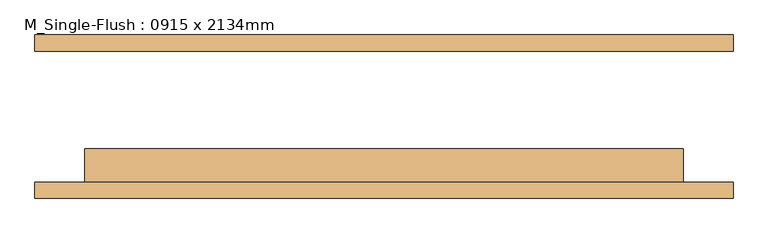
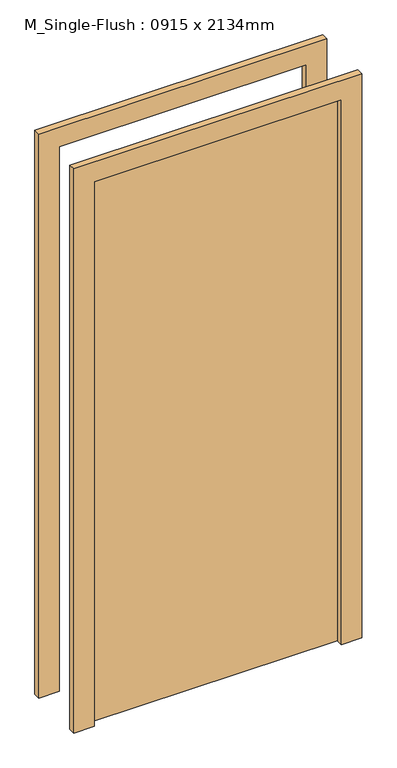
"""IFC4 building model written with IfcOpenShell, lengths in millimetres: door geometry, M_Single-Flush : 0915 x 2134mm."""

from ifc_helpers import new_model, si_unit, frame, origin, origin_with_axes, place, context, project, spatial, polyline, outline, extrude, source, transform, mapped, element, save


def m_single_flush_0915_x_2134mm_727434cd(model_context):
    return source(origin(), model_context, "Body", "SweptSolid", [
        extrude(outline(polyline([(2210.0, -533.5), (0.0, -533.5), (0.0, -457.5), (2134.0, -457.5), (2134.0, 457.5), (0.0, 457.5), (0.0, 533.5), (2210.0, 533.5), (2210.0, -533.5)])), frame((0.0, -125.0, 0.0), z_axis=(0.0, 1.0, 0.0), x_axis=(0.0, 0.0, 1.0)), (0.0, 0.0, 1.0), 25.0),
        extrude(outline(polyline([(2210.0, 533.5), (2210.0, -533.5), (0.0, -533.5), (0.0, -457.5), (2134.0, -457.5), (2134.0, 457.5), (0.0, 457.5), (0.0, 533.5), (2210.0, 533.5)])), frame((0.0, 100.0, 0.0), z_axis=(0.0, 1.0, 0.0), x_axis=(0.0, 0.0, 1.0)), (0.0, 0.0, 1.0), 25.0),
        extrude(outline(polyline([(457.5, -49.0), (457.5, -100.0), (-457.5, -100.0), (-457.5, -49.0), (457.5, -49.0)])), origin_with_axes(), (0.0, 0.0, 1.0), 2134.0),
    ])


if __name__ == "__main__":
    model = new_model("IFC4")
    model_context = context("Model", 3, world=origin())
    ifc_project = project(units=[si_unit("LENGTHUNIT", "METRE", prefix="MILLI")], contexts=[model_context])
    site = spatial("IfcSite", under=ifc_project)
    building = spatial("IfcBuilding", under=site)
    placement = place(None, origin())
    m_single_flush_0915_x_2134mm_shape = m_single_flush_0915_x_2134mm_727434cd(model_context)
    element("IfcDoor", 1, ObjectType="M_Single-Flush : 0915 x 2134mm", at=placement, inside=building, context=model_context, shape_type="MappedRepresentation", body=[
        mapped(m_single_flush_0915_x_2134mm_shape, transform((0.0, 0.0, 0.0), x_axis=(1.0, 0.0, 0.0), y_axis=(0.0, 1.0, 0.0), z_axis=(0.0, 0.0, 1.0))),
    ])
    save(model, "model.ifc")

# Revit data of these elements
# Type "M_Single-Flush : 0915 x 2134mm"
#   Type Mark = "15"
#   Thickness = 0' - 2.00787"
#   Height = 7' - 0.01575"
#   Trim Projection Ext = 0' - 0.98425"
#   Trim Projection Int = 0' - 0.98425"
#   Trim Width = 0' - 2.99213"
#   Width = 3' - 0.02362"
#   Door Material = Door - Panel
#   Frame Material = Door - Frame
#   Function = (empty or 0)
#   Wall Closure = (empty or 0)
# Element 1 (IfcDoor, "M_Single-Flush : 0915 x 2134mm")
#   Materials on its faces: "Door - Frame", "Door - Panel"
# Materials
#   "Door - Panel": class "Wood", colour RGB 114 82 51, transparency 0
#   "Door - Frame": colour RGB 153 76 43, transparency 0
